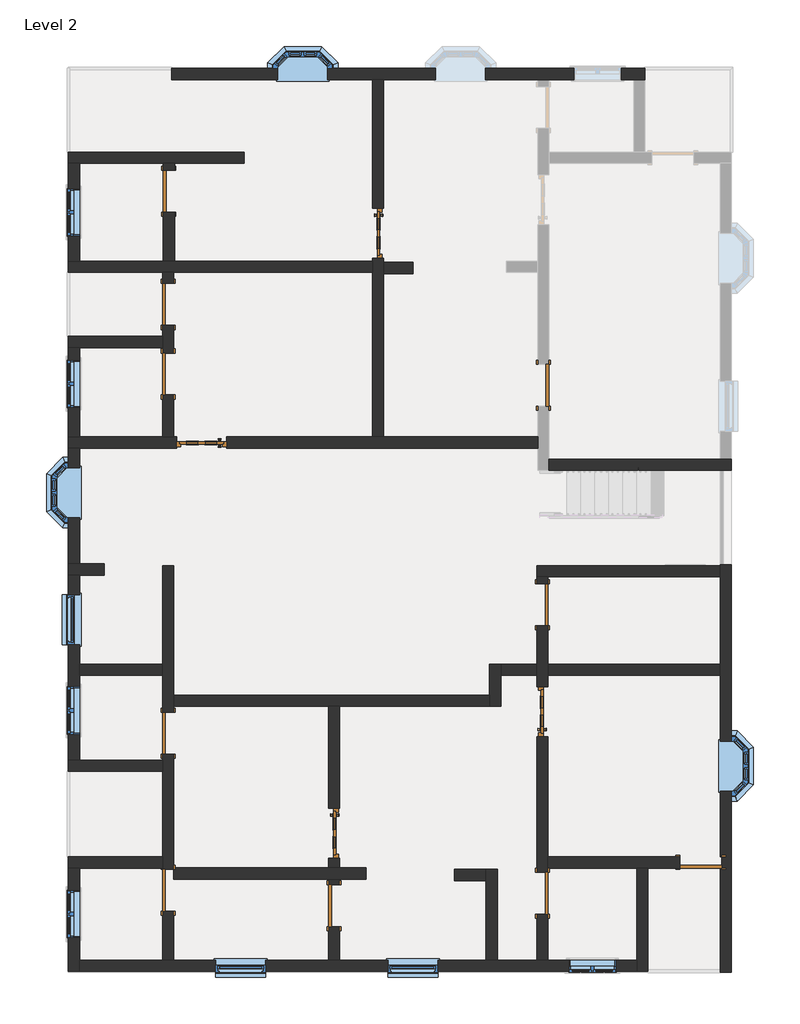
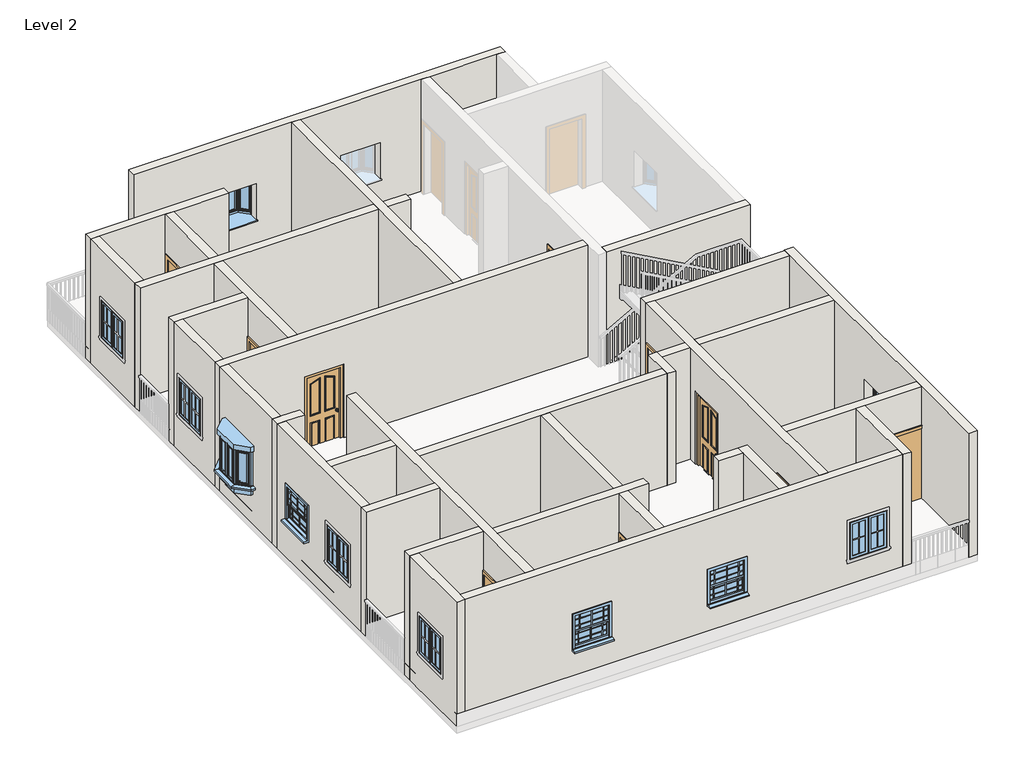
# One storey, part 1 of 4: 34 walls, 14 doors, 11 windows.
"""IFC4 building model written with IfcOpenShell, lengths in millimetres."""

from ifc_helpers import new_model, si_unit, frame, origin, place, context, project, spatial, polyline, outline, extrude, faceted_brep, transform, mapped, element, save
from components import doors_extsgl_12_910x2110mm_9a09825e, door_fadea3f2, door_53b1b562, window_910x910mm_67ef725a, window_c29befe5, windows_sash_w_bars_1_910x910mm_b688f793

model = new_model("IFC4")

# Units and contexts
model_context = context("Model", 3, world=origin())
ifc_project = project(units=[si_unit("LENGTHUNIT", "METRE", prefix="MILLI")], contexts=[model_context])

# Site, building, storey
site = spatial("IfcSite", under=ifc_project)
building = spatial("IfcBuilding", under=site)
storey = spatial("IfcBuildingStorey", under=building, Name="Level 2", Elevation=3048.0)

# Doors
placement = place(None, origin())
doors_extsgl_12_910x2110mm_shape = doors_extsgl_12_910x2110mm_9a09825e(model_context)
element("IfcDoor", 1, ObjectType="Doors_ExtSgl_12 : 910x2110mm", at=placement, inside=storey, context=model_context, shape_type="MappedRepresentation", body=[
    mapped(doors_extsgl_12_910x2110mm_shape, transform((-1409.2058717, 5320.2339901, 3048.0), x_axis=(0.0, -1.0, 0.0), y_axis=(1.0, 0.0, 0.0), z_axis=(0.0, 0.0, 1.0))),
])
element("IfcDoor", 2, ObjectType="Doors_ExtSgl_12 : 910x2110mm", at=placement, inside=storey, context=model_context, shape_type="MappedRepresentation", body=[
    mapped(doors_extsgl_12_910x2110mm_shape, transform((-4622.3058717, 1514.4547293, 3048.0), x_axis=(-1.0, 0.0, 0.0), y_axis=(0.0, -1.0, 0.0), z_axis=(0.0, 0.0, 1.0))),
])
element("IfcDoor", 3, ObjectType="Doors_ExtSgl_12 : 910x2110mm", at=placement, inside=storey, context=model_context, shape_type="MappedRepresentation", body=[
    mapped(doors_extsgl_12_910x2110mm_shape, transform((-2209.3058717, -5597.5452707, 3048.0), x_axis=(0.0, -1.0, 0.0), y_axis=(1.0, 0.0, 0.0), z_axis=(0.0, 0.0, 1.0))),
])
element("IfcDoor", 4, ObjectType="Doors_ExtSgl_12 : 910x2110mm", at=placement, inside=storey, context=model_context, shape_type="MappedRepresentation", body=[
    mapped(doors_extsgl_12_910x2110mm_shape, transform((1587.9941283, -3384.0437545, 3048.0), x_axis=(0.0, 1.0, 0.0), y_axis=(-1.0, 0.0, 0.0), z_axis=(0.0, 0.0, 1.0))),
])
door_shape = door_fadea3f2(model_context)
element("IfcDoor", 5, ObjectType="Single-Flush : 30\" x 80\"", at=placement, inside=storey, context=model_context, shape_type="MappedRepresentation", body=[
    mapped(door_shape, transform((-5219.2058717, 6086.4547293, 3048.0), x_axis=(0.0, 1.0, 0.0), y_axis=(-1.0, 0.0, 0.0), z_axis=(0.0, 0.0, 1.0))),
])
element("IfcDoor", 6, ObjectType="Single-Flush : 30\" x 80\"", at=placement, inside=storey, context=model_context, shape_type="MappedRepresentation", body=[
    mapped(door_shape, transform((-5231.9058717, -6637.2703483, 3048.0), x_axis=(0.0, 1.0, 0.0), y_axis=(-1.0, 0.0, 0.0), z_axis=(0.0, 0.0, 1.0))),
])
element("IfcDoor", 7, ObjectType="Single-Flush : 30\" x 80\"", at=placement, inside=storey, context=model_context, shape_type="MappedRepresentation", body=[
    mapped(door_shape, transform((-2209.3058717, -6918.3452707, 3048.0), x_axis=(0.0, 1.0, 0.0), y_axis=(-1.0, 0.0, 0.0), z_axis=(0.0, 0.0, 1.0))),
])
door_2_shape = door_53b1b562(model_context)
element("IfcDoor", 8, ObjectType="Single-Flush : 30\" x 80\"", at=placement, inside=storey, context=model_context, shape_type="MappedRepresentation", body=[
    mapped(door_2_shape, transform((-5231.9058717, 2759.0547293, 3048.0), x_axis=(0.0, -1.0, 0.0), y_axis=(1.0, 0.0, 0.0), z_axis=(0.0, 0.0, 1.0))),
])
element("IfcDoor", 9, ObjectType="Single-Flush : 30\" x 80\"", at=placement, inside=storey, context=model_context, shape_type="MappedRepresentation", body=[
    mapped(door_2_shape, transform((-5231.9058717, -3778.816952, 3048.0), x_axis=(0.0, -1.0, 0.0), y_axis=(1.0, 0.0, 0.0), z_axis=(0.0, 0.0, 1.0))),
])
element("IfcDoor", 10, ObjectType="Single-Flush : 30\" x 80\"", at=placement, inside=storey, context=model_context, shape_type="MappedRepresentation", body=[
    mapped(door_2_shape, transform((1587.9941283, -6689.7452707, 3048.0), x_axis=(0.0, 1.0, 0.0), y_axis=(-1.0, 0.0, 0.0), z_axis=(0.0, 0.0, 1.0))),
])
element("IfcDoor", 11, ObjectType="Single-Flush : 30\" x 80\"", at=placement, inside=storey, context=model_context, shape_type="MappedRepresentation", body=[
    mapped(door_2_shape, transform((4470.8941283, -6130.9452707, 3048.0), x_axis=(1.0, 0.0, 0.0), y_axis=(0.0, 1.0, 0.0), z_axis=(0.0, 0.0, 1.0))),
])
element("IfcDoor", 12, ObjectType="Single-Flush : 30\" x 80\"", at=placement, inside=storey, context=model_context, shape_type="MappedRepresentation", body=[
    mapped(door_2_shape, transform((1587.9941283, -1440.3867138, 3048.0), x_axis=(0.0, 1.0, 0.0), y_axis=(-1.0, 0.0, 0.0), z_axis=(0.0, 0.0, 1.0))),
])
element("IfcDoor", 13, ObjectType="Single-Flush : 30\" x 80\"", at=placement, inside=storey, context=model_context, shape_type="MappedRepresentation", body=[
    mapped(door_2_shape, transform((1600.6941283, 2555.8547293, 3048.0), x_axis=(0.0, 1.0, 0.0), y_axis=(-1.0, 0.0, 0.0), z_axis=(0.0, 0.0, 1.0))),
])
element("IfcDoor", 14, ObjectType="Single-Flush : 30\" x 80\"", at=placement, inside=storey, context=model_context, shape_type="MappedRepresentation", body=[
    mapped(door_2_shape, transform((-5231.9058717, 4026.9443597, 3048.0), x_axis=(0.0, -1.0, 0.0), y_axis=(1.0, 0.0, 0.0), z_axis=(0.0, 0.0, 1.0))),
])

# Walls
element("IfcWall", 15, ObjectType="Generic - 4.5\"", at=placement, inside=storey, context=model_context, shape_type="Brep", body=[
    faceted_brep([(-1510.8058717, 4865.2339901, 5158.0), (-1510.8058717, 4865.2339901, 3048.0), (-1510.8058717, 4812.2339901, 3048.0), (-1510.8058717, 4609.0339901, 3048.0), (-1510.8058717, 1616.0547293, 3048.0), (-1510.8058717, 1616.0547293, 6096.0), (-1510.8058717, 4609.0339901, 6096.0), (-1510.8058717, 4812.2339901, 6096.0), (-1510.8058717, 8118.4547293, 6096.0), (-1510.8058717, 8118.4547293, 3048.0), (-1510.8058717, 5775.2339901, 3048.0), (-1510.8058717, 5775.2339901, 5158.0), (-1307.6058717, 1616.0547293, 3048.0), (-1307.6058717, 4587.8547293, 3048.0), (-1307.6058717, 4791.0547293, 3048.0), (-1307.6058717, 4865.2339901, 3048.0), (-1307.6058717, 4865.2339901, 5158.0), (-1307.6058717, 5775.2339901, 5158.0), (-1307.6058717, 5775.2339901, 3048.0), (-1307.6058717, 8118.4547293, 3048.0), (-1307.6058717, 8118.4547293, 6096.0), (-1307.6058717, 4791.0547293, 6096.0), (-1307.6058717, 4587.8547293, 6096.0), (-1307.6058717, 1616.0547293, 6096.0)], [[[0, 1, 2, 3, 4, 5, 6, 7, 8, 9, 10, 11]], [[12, 13, 14, 15, 16, 17, 18, 19, 20, 21, 22, 23]], [[10, 9, 19, 18]], [[4, 3, 2, 1, 15, 14, 13, 12]], [[8, 7, 6, 5, 23, 22, 21, 20]], [[9, 8, 20, 19]], [[5, 4, 12, 23]], [[18, 17, 11, 10]], [[16, 15, 1, 0]], [[17, 16, 0, 11]]]),
])
element("IfcWall", 16, ObjectType="Generic - 4.5\"", at=placement, inside=storey, context=model_context, shape_type="Brep", body=[
    faceted_brep([(-7048.0058717, 4609.0339901, 3048.0), (-5333.5058717, 4609.0339901, 3048.0), (-5130.3058717, 4609.0339901, 3048.0), (-1510.8058717, 4609.0339901, 3048.0), (-1510.8058717, 4609.0339901, 6096.0), (-5130.3058717, 4609.0339901, 6096.0), (-5333.5058717, 4609.0339901, 6096.0), (-7048.0058717, 4609.0339901, 6096.0), (-7048.0058717, 4812.2339901, 3048.0), (-7048.0058717, 4812.2339901, 6096.0), (-6844.8058717, 4812.2339901, 6096.0), (-5320.8058717, 4812.2339901, 6096.0), (-5117.6058717, 4812.2339901, 6096.0), (-1510.8058717, 4812.2339901, 6096.0), (-1510.8058717, 4812.2339901, 3048.0), (-5117.6058717, 4812.2339901, 3048.0), (-5320.8058717, 4812.2339901, 3048.0), (-6844.8058717, 4812.2339901, 3048.0)], [[[0, 1, 2, 3, 4, 5, 6, 7]], [[8, 9, 10, 11, 12, 13, 14, 15, 16, 17]], [[3, 2, 1, 0, 8, 17, 16, 15, 14]], [[7, 6, 5, 4, 13, 12, 11, 10, 9]], [[4, 3, 14, 13]], [[0, 7, 9, 8]]]),
])
element("IfcWall", 17, ObjectType="Generic - 4.5\"", at=placement, inside=storey, context=model_context, shape_type="Brep", body=[
    faceted_brep([(-5333.5058717, 3645.9443597, 5080.0), (-5333.5058717, 3645.9443597, 3048.0), (-5333.5058717, 3444.8547293, 3048.0), (-5333.5058717, 3241.6547293, 3048.0), (-5333.5058717, 3140.0547293, 3048.0), (-5333.5058717, 3140.0547293, 5080.0), (-5333.5058717, 2378.0547293, 5080.0), (-5333.5058717, 2378.0547293, 3048.0), (-5333.5058717, 1616.0547293, 3048.0), (-5333.5058717, 1616.0547293, 6096.0), (-5333.5058717, 3241.6547293, 6096.0), (-5333.5058717, 3444.8547293, 6096.0), (-5333.5058717, 4609.0339901, 6096.0), (-5333.5058717, 4609.0339901, 3048.0), (-5333.5058717, 4407.9443597, 3048.0), (-5333.5058717, 4407.9443597, 5080.0), (-5130.3058717, 3140.0547293, 3048.0), (-5130.3058717, 3645.9443597, 3048.0), (-5130.3058717, 3645.9443597, 5080.0), (-5130.3058717, 4407.9443597, 5080.0), (-5130.3058717, 4407.9443597, 3048.0), (-5130.3058717, 4609.0339901, 3048.0), (-5130.3058717, 4609.0339901, 6096.0), (-5130.3058717, 1616.0547293, 6096.0), (-5130.3058717, 1616.0547293, 3048.0), (-5130.3058717, 2378.0547293, 3048.0), (-5130.3058717, 2378.0547293, 5080.0), (-5130.3058717, 3140.0547293, 5080.0)], [[[0, 1, 2, 3, 4, 5, 6, 7, 8, 9, 10, 11, 12, 13, 14, 15]], [[16, 17, 18, 19, 20, 21, 22, 23, 24, 25, 26, 27]], [[8, 7, 25, 24]], [[14, 13, 21, 20]], [[4, 3, 2, 1, 17, 16]], [[12, 11, 10, 9, 23, 22]], [[13, 12, 22, 21]], [[9, 8, 24, 23]], [[26, 25, 7, 6]], [[27, 26, 6, 5]], [[16, 27, 5, 4]], [[18, 17, 1, 0]], [[19, 18, 0, 15]], [[20, 19, 15, 14]]]),
])
element("IfcWall", 18, ObjectType="Generic - 4.5\"", at=placement, inside=storey, context=model_context, shape_type="Brep", body=[
    faceted_brep([(-5130.3058717, -6256.2703483, 5080.0), (-5130.3058717, -6256.2703483, 3048.0), (-5130.3058717, -6230.8703483, 3048.0), (-5130.3058717, -4159.816952, 3048.0), (-5130.3058717, -4159.816952, 5080.0), (-5130.3058717, -3397.816952, 5080.0), (-5130.3058717, -3397.816952, 3048.0), (-5130.3058717, -3286.1452707, 3048.0), (-5130.3058717, -3082.9452707, 3048.0), (-5130.3058717, -733.4452707, 3048.0), (-5130.3058717, -733.4452707, 6096.0), (-5130.3058717, -3082.9452707, 6096.0), (-5130.3058717, -3286.1452707, 6096.0), (-5130.3058717, -6230.8703483, 6096.0), (-5130.3058717, -6434.0703483, 6096.0), (-5130.3058717, -7908.9452707, 6096.0), (-5130.3058717, -7908.9452707, 3048.0), (-5130.3058717, -7018.2703483, 3048.0), (-5130.3058717, -7018.2703483, 5080.0), (-5333.5058717, -4159.816952, 3048.0), (-5333.5058717, -4271.4886333, 3048.0), (-5333.5058717, -4474.6886333, 3048.0), (-5333.5058717, -6029.3452707, 3048.0), (-5333.5058717, -6232.5452707, 3048.0), (-5333.5058717, -6256.2703483, 3048.0), (-5333.5058717, -6256.2703483, 5080.0), (-5333.5058717, -7018.2703483, 5080.0), (-5333.5058717, -7018.2703483, 3048.0), (-5333.5058717, -7908.9452707, 3048.0), (-5333.5058717, -7908.9452707, 6096.0), (-5333.5058717, -6232.5452707, 6096.0), (-5333.5058717, -6029.3452707, 6096.0), (-5333.5058717, -4474.6886333, 6096.0), (-5333.5058717, -4271.4886333, 6096.0), (-5333.5058717, -2727.3452707, 6096.0), (-5333.5058717, -2524.1452707, 6096.0), (-5333.5058717, -733.4452707, 6096.0), (-5333.5058717, -733.4452707, 3048.0), (-5333.5058717, -2524.1452707, 3048.0), (-5333.5058717, -2727.3452707, 3048.0), (-5333.5058717, -3397.816952, 3048.0), (-5333.5058717, -3397.816952, 5080.0), (-5333.5058717, -4159.816952, 5080.0)], [[[0, 1, 2, 3, 4, 5, 6, 7, 8, 9, 10, 11, 12, 13, 14, 15, 16, 17, 18]], [[19, 20, 21, 22, 23, 24, 25, 26, 27, 28, 29, 30, 31, 32, 33, 34, 35, 36, 37, 38, 39, 40, 41, 42]], [[40, 39, 38, 37, 9, 8, 7, 6]], [[17, 16, 28, 27]], [[3, 2, 1, 24, 23, 22, 21, 20, 19]], [[10, 9, 37, 36]], [[15, 14, 13, 12, 11, 10, 36, 35, 34, 33, 32, 31, 30, 29]], [[4, 3, 19, 42]], [[5, 4, 42, 41]], [[6, 5, 41, 40]], [[25, 24, 1, 0]], [[26, 25, 0, 18]], [[27, 26, 18, 17]], [[16, 15, 29, 28]]]),
])
element("IfcWall", 19, ObjectType="Generic - 4.5\"", at=placement, inside=storey, context=model_context, shape_type="Brep", body=[
    faceted_brep([(-7048.0058717, -898.5452707, 3048.0), (-6844.8058717, -898.5452707, 3048.0), (-6400.7404065, -898.5452707, 3048.0), (-6400.7404065, -898.5452707, 6096.0), (-6844.8058717, -898.5452707, 6096.0), (-7048.0058717, -898.5452707, 6096.0), (-7048.0058717, -695.3452707, 3048.0), (-7048.0058717, -695.3452707, 6096.0), (-6844.8058717, -695.3452707, 6096.0), (-6400.7404065, -695.3452707, 6096.0), (-6400.7404065, -695.3452707, 3048.0), (-6844.8058717, -695.3452707, 3048.0)], [[[0, 1, 2, 3, 4, 5]], [[6, 7, 8, 9, 10, 11]], [[2, 1, 0, 6, 11, 10]], [[3, 2, 10, 9]], [[5, 4, 3, 9, 8, 7]], [[0, 5, 7, 6]]]),
])
element("IfcWall", 20, ObjectType="Generic - 4.5\"", at=placement, inside=storey, context=model_context, shape_type="Brep", body=[
    faceted_brep([(-7048.0058717, 6594.4547293, 3048.0), (-6844.8058717, 6594.4547293, 3048.0), (-5320.8058717, 6594.4547293, 3048.0), (-5117.6058717, 6594.4547293, 3048.0), (-3847.6058717, 6594.4547293, 3048.0), (-3847.6058717, 6594.4547293, 6096.0), (-5117.6058717, 6594.4547293, 6096.0), (-5320.8058717, 6594.4547293, 6096.0), (-6844.8058717, 6594.4547293, 6096.0), (-7048.0058717, 6594.4547293, 6096.0), (-7048.0058717, 6797.6547293, 3048.0), (-7048.0058717, 6797.6547293, 6096.0), (-3847.6058717, 6797.6547293, 6096.0), (-3847.6058717, 6797.6547293, 3048.0)], [[[0, 1, 2, 3, 4, 5, 6, 7, 8, 9]], [[10, 11, 12, 13]], [[4, 3, 2, 1, 0, 10, 13]], [[5, 4, 13, 12]], [[9, 8, 7, 6, 5, 12, 11]], [[0, 9, 11, 10]]]),
])
element("IfcWall", 21, ObjectType="Generic - 4.5\"", at=placement, inside=storey, context=model_context, shape_type="Brep", body=[
    faceted_brep([(-7048.0058717, 3241.6547293, 3048.0), (-6844.8058717, 3241.6547293, 3048.0), (-5333.5058717, 3241.6547293, 3048.0), (-5333.5058717, 3241.6547293, 6096.0), (-6844.8058717, 3241.6547293, 6096.0), (-7048.0058717, 3241.6547293, 6096.0), (-7048.0058717, 3444.8547293, 3048.0), (-7048.0058717, 3444.8547293, 6096.0), (-5333.5058717, 3444.8547293, 6096.0), (-5333.5058717, 3444.8547293, 3048.0)], [[[0, 1, 2, 3, 4, 5]], [[6, 7, 8, 9]], [[2, 1, 0, 6, 9]], [[5, 4, 3, 8, 7]], [[3, 2, 9, 8]], [[0, 5, 7, 6]]]),
])
element("IfcWall", 22, ObjectType="Generic - 4.5\"", at=placement, inside=storey, context=model_context, shape_type="Brep", body=[
    faceted_brep([(-7048.0058717, 1412.8547293, 3048.0), (-6844.8058717, 1412.8547293, 3048.0), (-5077.3058717, 1412.8547293, 3048.0), (-5077.3058717, 1412.8547293, 5158.0), (-4167.3058717, 1412.8547293, 5158.0), (-4167.3058717, 1412.8547293, 3048.0), (1499.0941283, 1412.8547293, 3048.0), (1499.0941283, 1412.8547293, 6096.0), (-6844.8058717, 1412.8547293, 6096.0), (-7048.0058717, 1412.8547293, 6096.0), (-5077.3058717, 1616.0547293, 5158.0), (-5077.3058717, 1616.0547293, 3048.0), (-5130.3058717, 1616.0547293, 3048.0), (-5333.5058717, 1616.0547293, 3048.0), (-6844.8058717, 1616.0547293, 3048.0), (-7048.0058717, 1616.0547293, 3048.0), (-7048.0058717, 1616.0547293, 6096.0), (-6844.8058717, 1616.0547293, 6096.0), (-5333.5058717, 1616.0547293, 6096.0), (-5130.3058717, 1616.0547293, 6096.0), (-1510.8058717, 1616.0547293, 6096.0), (-1307.6058717, 1616.0547293, 6096.0), (1499.0941283, 1616.0547293, 6096.0), (1499.0941283, 1616.0547293, 3048.0), (-1307.6058717, 1616.0547293, 3048.0), (-1510.8058717, 1616.0547293, 3048.0), (-4167.3058717, 1616.0547293, 3048.0), (-4167.3058717, 1616.0547293, 5158.0)], [[[0, 1, 2, 3, 4, 5, 6, 7, 8, 9]], [[10, 11, 12, 13, 14, 15, 16, 17, 18, 19, 20, 21, 22, 23, 24, 25, 26, 27]], [[26, 25, 24, 23, 6, 5]], [[15, 14, 13, 12, 11, 2, 1, 0]], [[9, 8, 7, 22, 21, 20, 19, 18, 17, 16]], [[7, 6, 23, 22]], [[5, 4, 27, 26]], [[3, 2, 11, 10]], [[4, 3, 10, 27]], [[0, 9, 16, 15]]]),
])
element("IfcWall", 23, ObjectType="Generic - 4.5\"", at=placement, inside=storey, context=model_context, shape_type="Brep", body=[
    faceted_brep([(1702.2941283, 1006.4547293, 3048.0), (5029.6941283, 1006.4547293, 3048.0), (5029.6941283, 1006.4547293, 6096.0), (1702.2941283, 1006.4547293, 6096.0), (1702.2941283, 1209.6547293, 3048.0), (1702.2941283, 1209.6547293, 6096.0), (4826.4941283, 1209.6547293, 6096.0), (5029.6941283, 1209.6547293, 6096.0), (5029.6941283, 1209.6547293, 3048.0), (4826.4941283, 1209.6547293, 3048.0)], [[[0, 1, 2, 3]], [[4, 5, 6, 7, 8, 9]], [[1, 0, 4, 9, 8]], [[3, 2, 7, 6, 5]], [[0, 3, 5, 4]], [[2, 1, 8, 7]]]),
])
element("IfcWall", 24, ObjectType="Generic - 4.5\"", at=placement, inside=storey, context=model_context, shape_type="Brep", body=[
    faceted_brep([(1486.3941283, -932.3867138, 3048.0), (1689.5941283, -932.3867138, 3048.0), (4826.4941283, -932.3867138, 3048.0), (4826.4941283, -932.3867138, 6096.0), (1689.5941283, -932.3867138, 6096.0), (1486.3941283, -932.3867138, 6096.0), (1486.3941283, -729.1867138, 3048.0), (1486.3941283, -729.1867138, 6096.0), (4826.4941283, -729.1867138, 6096.0), (4826.4941283, -729.1867138, 3048.0)], [[[0, 1, 2, 3, 4, 5]], [[6, 7, 8, 9]], [[2, 1, 0, 6, 9]], [[5, 4, 3, 8, 7]], [[3, 2, 9, 8]], [[0, 5, 7, 6]]]),
])
element("IfcWall", 25, ObjectType="Generic - 4.5\"", at=placement, inside=storey, context=model_context, shape_type="Brep", body=[
    faceted_brep([(1486.3941283, -932.3867138, 3048.0), (1486.3941283, -1059.3867138, 3048.0), (1486.3941283, -1059.3867138, 5080.0), (1486.3941283, -1821.3867138, 5080.0), (1486.3941283, -1821.3867138, 3048.0), (1486.3941283, -2520.4437545, 3048.0), (1486.3941283, -2723.6437545, 3048.0), (1486.3941283, -2929.0437545, 3048.0), (1486.3941283, -2929.0437545, 5158.0), (1486.3941283, -3839.0437545, 5158.0), (1486.3941283, -3839.0437545, 3048.0), (1486.3941283, -6308.7452707, 3048.0), (1486.3941283, -6308.7452707, 5080.0), (1486.3941283, -7070.7452707, 5080.0), (1486.3941283, -7070.7452707, 3048.0), (1486.3941283, -7908.9452707, 3048.0), (1486.3941283, -7908.9452707, 6096.0), (1486.3941283, -2723.6437545, 6096.0), (1486.3941283, -2520.4437545, 6096.0), (1486.3941283, -932.3867138, 6096.0), (1689.5941283, -1059.3867138, 5080.0), (1689.5941283, -1059.3867138, 3048.0), (1689.5941283, -932.3867138, 3048.0), (1689.5941283, -932.3867138, 6096.0), (1689.5941283, -2520.4437545, 6096.0), (1689.5941283, -2723.6437545, 6096.0), (1689.5941283, -6029.3452707, 6096.0), (1689.5941283, -6232.5452707, 6096.0), (1689.5941283, -7908.9452707, 6096.0), (1689.5941283, -7908.9452707, 3048.0), (1689.5941283, -7070.7452707, 3048.0), (1689.5941283, -7070.7452707, 5080.0), (1689.5941283, -6308.7452707, 5080.0), (1689.5941283, -6308.7452707, 3048.0), (1689.5941283, -6232.5452707, 3048.0), (1689.5941283, -6029.3452707, 3048.0), (1689.5941283, -3839.0437545, 3048.0), (1689.5941283, -3839.0437545, 5158.0), (1689.5941283, -2929.0437545, 5158.0), (1689.5941283, -2929.0437545, 3048.0), (1689.5941283, -2723.6437545, 3048.0), (1689.5941283, -2520.4437545, 3048.0), (1689.5941283, -1821.3867138, 3048.0), (1689.5941283, -1821.3867138, 5080.0)], [[[0, 1, 2, 3, 4, 5, 6, 7, 8, 9, 10, 11, 12, 13, 14, 15, 16, 17, 18, 19]], [[20, 21, 22, 23, 24, 25, 26, 27, 28, 29, 30, 31, 32, 33, 34, 35, 36, 37, 38, 39, 40, 41, 42, 43]], [[30, 29, 15, 14]], [[36, 35, 34, 33, 11, 10]], [[22, 21, 1, 0]], [[42, 41, 40, 39, 7, 6, 5, 4]], [[19, 18, 17, 16, 28, 27, 26, 25, 24, 23]], [[0, 19, 23, 22]], [[10, 9, 37, 36]], [[8, 7, 39, 38]], [[9, 8, 38, 37]], [[12, 11, 33, 32]], [[13, 12, 32, 31]], [[14, 13, 31, 30]], [[2, 1, 21, 20]], [[3, 2, 20, 43]], [[4, 3, 43, 42]], [[16, 15, 29, 28]]]),
])
element("IfcWall", 26, ObjectType="Generic - 4.5\"", at=placement, inside=storey, context=model_context, shape_type="SweptSolid", body=[
    extrude(outline(polyline([(4826.4941283, -2723.6437545), (1689.5941283, -2723.6437545), (1689.5941283, -2520.4437545), (4826.4941283, -2520.4437545), (4826.4941283, -2723.6437545)])), frame((0.0, 0.0, 3048.0), z_axis=(0.0, 0.0, 1.0), x_axis=(1.0, 0.0, 0.0)), (0.0, 0.0, 1.0), 3048.0),
])
element("IfcWall", 27, ObjectType="Generic - 4.5\"", at=placement, inside=storey, context=model_context, shape_type="Brep", body=[
    faceted_brep([(4826.4941283, -6232.5452707, 6096.0), (3505.6941283, -6232.5452707, 6096.0), (3302.4941283, -6232.5452707, 6096.0), (1689.5941283, -6232.5452707, 6096.0), (1689.5941283, -6232.5452707, 3048.0), (3302.4941283, -6232.5452707, 3048.0), (3505.6941283, -6232.5452707, 3048.0), (4089.8941283, -6232.5452707, 3048.0), (4089.8941283, -6232.5452707, 5080.0), (4826.4941283, -6232.5452707, 5080.0), (1689.5941283, -6029.3452707, 6096.0), (4826.4941283, -6029.3452707, 6096.0), (4826.4941283, -6029.3452707, 5080.0), (4089.8941283, -6029.3452707, 5080.0), (4089.8941283, -6029.3452707, 3048.0), (1689.5941283, -6029.3452707, 3048.0)], [[[0, 1, 2, 3, 4, 5, 6, 7, 8, 9]], [[10, 11, 12, 13, 14, 15]], [[4, 15, 14, 7, 6, 5]], [[3, 2, 1, 0, 11, 10]], [[11, 0, 9, 12]], [[4, 3, 10, 15]], [[8, 13, 12, 9]], [[13, 8, 7, 14]]]),
])
element("IfcWall", 28, ObjectType="Generic - 4.5\"", at=placement, inside=storey, context=model_context, shape_type="Brep", body=[
    faceted_brep([(3302.4941283, -6232.5452707, 3048.0), (3302.4941283, -7908.9452707, 3048.0), (3302.4941283, -8112.1452707, 3048.0), (3302.4941283, -8112.1452707, 6096.0), (3302.4941283, -7908.9452707, 6096.0), (3302.4941283, -6232.5452707, 6096.0), (3505.6941283, -6232.5452707, 3048.0), (3505.6941283, -6232.5452707, 6096.0), (3505.6941283, -8112.1452707, 6096.0), (3505.6941283, -8112.1452707, 3048.0)], [[[0, 1, 2, 3, 4, 5]], [[6, 7, 8, 9]], [[2, 1, 0, 6, 9]], [[5, 4, 3, 8, 7]], [[0, 5, 7, 6]], [[3, 2, 9, 8]]]),
])
element("IfcWall", 29, ObjectType="Generic - 4.5\"", at=placement, inside=storey, context=model_context, shape_type="SweptSolid", body=[
    extrude(outline(polyline([(-5333.5058717, -2727.3452707), (-6844.8058717, -2727.3452707), (-6844.8058717, -2524.1452707), (-5333.5058717, -2524.1452707), (-5333.5058717, -2727.3452707)])), frame((0.0, 0.0, 3048.0), z_axis=(0.0, 0.0, 1.0), x_axis=(1.0, 0.0, 0.0)), (0.0, 0.0, 1.0), 3048.0),
])
element("IfcWall", 30, ObjectType="Generic - 4.5\"", at=placement, inside=storey, context=model_context, shape_type="Brep", body=[
    faceted_brep([(-7048.0058717, -4474.6886333, 3048.0), (-5333.5058717, -4474.6886333, 3048.0), (-5333.5058717, -4474.6886333, 6096.0), (-7048.0058717, -4474.6886333, 6096.0), (-7048.0058717, -4271.4886333, 3048.0), (-7048.0058717, -4271.4886333, 6096.0), (-6844.8058717, -4271.4886333, 6096.0), (-5333.5058717, -4271.4886333, 6096.0), (-5333.5058717, -4271.4886333, 3048.0), (-6844.8058717, -4271.4886333, 3048.0)], [[[0, 1, 2, 3]], [[4, 5, 6, 7, 8, 9]], [[1, 0, 4, 9, 8]], [[3, 2, 7, 6, 5]], [[2, 1, 8, 7]], [[0, 3, 5, 4]]]),
])
element("IfcWall", 31, ObjectType="Generic - 4.5\"", at=placement, inside=storey, context=model_context, shape_type="Brep", body=[
    faceted_brep([(-7048.0058717, -6232.5452707, 3048.0), (-6844.8058717, -6232.5452707, 3048.0), (-5333.5058717, -6232.5452707, 3048.0), (-5333.5058717, -6232.5452707, 6096.0), (-6844.8058717, -6232.5452707, 6096.0), (-7048.0058717, -6232.5452707, 6096.0), (-7048.0058717, -6029.3452707, 3048.0), (-7048.0058717, -6029.3452707, 6096.0), (-5333.5058717, -6029.3452707, 6096.0), (-5333.5058717, -6029.3452707, 3048.0)], [[[0, 1, 2, 3, 4, 5]], [[6, 7, 8, 9]], [[2, 1, 0, 6, 9]], [[5, 4, 3, 8, 7]], [[3, 2, 9, 8]], [[0, 5, 7, 6]]]),
])
element("IfcWall", 32, ObjectType="Generic - 4.5\"", at=placement, inside=storey, context=model_context, shape_type="Brep", body=[
    faceted_brep([(-5130.3058717, -6434.0703483, 3048.0), (-2310.9058717, -6434.0703483, 3048.0), (-2107.7058717, -6434.0703483, 3048.0), (-1625.1058717, -6434.0703483, 3048.0), (-1625.1058717, -6434.0703483, 6096.0), (-2107.7058717, -6434.0703483, 6096.0), (-2310.9058717, -6434.0703483, 6096.0), (-5130.3058717, -6434.0703483, 6096.0), (-5130.3058717, -6230.8703483, 3048.0), (-5130.3058717, -6230.8703483, 6096.0), (-2310.9058717, -6230.8703483, 6096.0), (-2107.7058717, -6230.8703483, 6096.0), (-1625.1058717, -6230.8703483, 6096.0), (-1625.1058717, -6230.8703483, 3048.0), (-2107.7058717, -6230.8703483, 3048.0), (-2310.9058717, -6230.8703483, 3048.0), (-5130.3058717, -6256.2703483, 3048.0)], [[[0, 1, 2, 3, 4, 5, 6, 7]], [[8, 9, 10, 11, 12, 13, 14, 15]], [[3, 2, 1, 0, 16, 8, 15, 14, 13]], [[4, 3, 13, 12]], [[7, 6, 5, 4, 12, 11, 10, 9]], [[0, 7, 9, 8, 16]]]),
])
element("IfcWall", 33, ObjectType="Generic - 4.5\"", at=placement, inside=storey, context=model_context, shape_type="Brep", body=[
    faceted_brep([(762.4941283, -7908.9452707, 3048.0), (762.4941283, -6257.9452707, 3048.0), (762.4941283, -6257.9452707, 6096.0), (762.4941283, -7908.9452707, 6096.0), (559.2941283, -7908.9452707, 3048.0), (559.2941283, -7908.9452707, 6096.0), (559.2941283, -6461.1452707, 6096.0), (559.2941283, -6257.9452707, 6096.0), (559.2941283, -6257.9452707, 3048.0), (559.2941283, -6461.1452707, 3048.0)], [[[0, 1, 2, 3]], [[4, 5, 6, 7, 8, 9]], [[1, 0, 4, 9, 8]], [[3, 2, 7, 6, 5]], [[2, 1, 8, 7]], [[0, 3, 5, 4]]]),
])
element("IfcWall", 34, ObjectType="Generic - 4.5\"", at=placement, inside=storey, context=model_context, shape_type="SweptSolid", body=[
    extrude(outline(polyline([(-12.2058717, -6257.9452707), (559.2941283, -6257.9452707), (559.2941283, -6461.1452707), (-12.2058717, -6461.1452707), (-12.2058717, -6257.9452707)])), frame((0.0, 0.0, 3048.0), z_axis=(0.0, 0.0, 1.0), x_axis=(1.0, 0.0, 0.0)), (0.0, 0.0, 1.0), 3048.0),
])
element("IfcWall", 35, ObjectType="Generic - 4.5\"", at=placement, inside=storey, context=model_context, shape_type="SweptSolid", body=[
    extrude(outline(polyline([(-3286.1452707, 6096.0), (-3286.1452707, 3048.0), (-5142.5452707, 3048.0), (-5142.5452707, 5158.0), (-6052.5452707, 5158.0), (-6052.5452707, 3048.0), (-6230.8703483, 3048.0), (-6230.8703483, 6096.0), (-3286.1452707, 6096.0)])), frame((-2310.9058717, 0.0, 0.0), z_axis=(1.0, 0.0, 0.0), x_axis=(0.0, 1.0, 0.0)), (0.0, 0.0, 1.0), 203.2),
    extrude(outline(polyline([(-6537.3452707, 3048.0), (-6537.3452707, 5080.0), (-7299.3452707, 5080.0), (-7299.3452707, 3048.0), (-7908.9452707, 3048.0), (-7908.9452707, 6096.0), (-6434.0703483, 6096.0), (-6434.0703483, 3048.0), (-6537.3452707, 3048.0)])), frame((-2310.9058717, 0.0, 0.0), z_axis=(1.0, 0.0, 0.0), x_axis=(0.0, 1.0, 0.0)), (0.0, 0.0, 1.0), 203.2),
])
element("IfcWall", 36, ObjectType="Generic - 4.5\"", at=placement, inside=storey, context=model_context, shape_type="Brep", body=[
    faceted_brep([(-5130.3058717, -3286.1452707, 3048.0), (-2310.9058717, -3286.1452707, 3048.0), (-2107.7058717, -3286.1452707, 3048.0), (622.0199378, -3286.1452707, 3048.0), (622.0199378, -3286.1452707, 6096.0), (-2107.7058717, -3286.1452707, 6096.0), (-2310.9058717, -3286.1452707, 6096.0), (-5130.3058717, -3286.1452707, 6096.0), (-5130.3058717, -3082.9452707, 3048.0), (-5130.3058717, -3082.9452707, 6096.0), (622.0199378, -3082.9452707, 6096.0), (622.0199378, -3082.9452707, 3048.0)], [[[0, 1, 2, 3, 4, 5, 6, 7]], [[8, 9, 10, 11]], [[3, 2, 1, 0, 8, 11]], [[7, 6, 5, 4, 10, 9]], [[0, 7, 9, 8]], [[4, 3, 11, 10]]]),
])
element("IfcWall", 37, ObjectType="Generic - 4.5\"", at=placement, inside=storey, context=model_context, shape_type="Brep", body=[
    faceted_brep([(825.2199378, -3286.1452707, 3048.0), (825.2199378, -2723.6437545, 3048.0), (825.2199378, -2520.4437545, 3048.0), (825.2199378, -2520.4437545, 6096.0), (825.2199378, -2723.6437545, 6096.0), (825.2199378, -3286.1452707, 6096.0), (622.0199378, -3286.1452707, 3048.0), (622.0199378, -3286.1452707, 6096.0), (622.0199378, -3082.9452707, 6096.0), (622.0199378, -2520.4437545, 6096.0), (622.0199378, -2520.4437545, 3048.0), (622.0199378, -3082.9452707, 3048.0)], [[[0, 1, 2, 3, 4, 5]], [[6, 7, 8, 9, 10, 11]], [[2, 1, 0, 6, 11, 10]], [[5, 4, 3, 9, 8, 7]], [[0, 5, 7, 6]], [[3, 2, 10, 9]]]),
])
element("IfcWall", 38, ObjectType="Generic - 4.5\"", at=placement, inside=storey, context=model_context, shape_type="SweptSolid", body=[
    extrude(outline(polyline([(1486.3941283, -2723.6437545), (825.2199378, -2723.6437545), (825.2199378, -2520.4437545), (1486.3941283, -2520.4437545), (1486.3941283, -2723.6437545)])), frame((0.0, 0.0, 3048.0), z_axis=(0.0, 0.0, 1.0), x_axis=(1.0, 0.0, 0.0)), (0.0, 0.0, 1.0), 3048.0),
])
element("IfcWall", 39, ObjectType="Generic - 4.5\"", at=placement, inside=storey, context=model_context, shape_type="SweptSolid", body=[
    extrude(outline(polyline([(-774.2058717, 4587.8547293), (-1307.6058717, 4587.8547293), (-1307.6058717, 4791.0547293), (-774.2058717, 4791.0547293), (-774.2058717, 4587.8547293)])), frame((0.0, 0.0, 3048.0), z_axis=(0.0, 0.0, 1.0), x_axis=(1.0, 0.0, 0.0)), (0.0, 0.0, 1.0), 3048.0),
])
element("IfcWall", 40, ObjectType="Generic - 4.5\"", at=placement, inside=storey, context=model_context, shape_type="SweptSolid", body=[
    extrude(outline(polyline([(6594.4547293, 3048.0), (6467.4547293, 3048.0), (6467.4547293, 5080.0), (5705.4547293, 5080.0), (5705.4547293, 3048.0), (4812.2339901, 3048.0), (4812.2339901, 6096.0), (6594.4547293, 6096.0), (6594.4547293, 3048.0)])), frame((-5320.8058717, 0.0, 0.0), z_axis=(1.0, 0.0, 0.0), x_axis=(0.0, 1.0, 0.0)), (0.0, 0.0, 1.0), 203.2),
])
element("IfcWall", 41, ObjectType="Generic - 9\"", at=placement, inside=storey, context=model_context, shape_type="Brep", body=[
    faceted_brep([(-5168.4058717, 8118.4547293, 3048.0), (-1510.8058717, 8118.4547293, 3048.0), (-1307.6058717, 8118.4547293, 3048.0), (1499.0941283, 8118.4547293, 3048.0), (1702.2941283, 8118.4547293, 3048.0), (3251.6941283, 8118.4547293, 3048.0), (3454.8941283, 8118.4547293, 3048.0), (3454.8941283, 8118.4547293, 6096.0), (3251.6941283, 8118.4547293, 6096.0), (1702.2941283, 8118.4547293, 6096.0), (1499.0941283, 8118.4547293, 6096.0), (-1307.6058717, 8118.4547293, 6096.0), (-1510.8058717, 8118.4547293, 6096.0), (-5168.4058717, 8118.4547293, 6096.0), (-359.2558717, 8118.4547293, 4872.4), (550.7441283, 8118.4547293, 4872.4), (550.7441283, 8118.4547293, 3962.4), (-359.2558717, 8118.4547293, 3962.4), (-3235.8058717, 8118.4547293, 4872.4), (-2325.8058717, 8118.4547293, 4872.4), (-2325.8058717, 8118.4547293, 3962.4), (-3235.8058717, 8118.4547293, 3962.4), (3023.0941283, 8118.4547293, 4876.8), (3023.0941283, 8118.4547293, 3962.4), (2159.4941283, 8118.4547293, 3962.4), (2159.4941283, 8118.4547293, 4876.8), (-5168.4058717, 8321.6547293, 3048.0), (-5168.4058717, 8321.6547293, 6096.0), (3454.8941283, 8321.6547293, 6096.0), (3454.8941283, 8321.6547293, 3048.0), (-359.2558717, 8321.6547293, 4872.4), (-359.2558717, 8321.6547293, 3962.4), (550.7441283, 8321.6547293, 3962.4), (550.7441283, 8321.6547293, 4872.4), (-3235.8058717, 8321.6547293, 4872.4), (-3235.8058717, 8321.6547293, 3962.4), (-2325.8058717, 8321.6547293, 3962.4), (-2325.8058717, 8321.6547293, 4872.4), (3023.0941283, 8321.6547293, 4876.8), (2159.4941283, 8321.6547293, 4876.8), (2159.4941283, 8321.6547293, 3962.4), (3023.0941283, 8321.6547293, 3962.4)], [[[0, 1, 2, 3, 4, 5, 6, 7, 8, 9, 10, 11, 12, 13], [14, 15, 16, 17], [18, 19, 20, 21], [22, 23, 24, 25]], [[26, 27, 28, 29], [30, 31, 32, 33], [34, 35, 36, 37], [38, 39, 40, 41]], [[6, 5, 4, 3, 2, 1, 0, 26, 29]], [[13, 12, 11, 10, 9, 8, 7, 28, 27]], [[0, 13, 27, 26]], [[31, 30, 14, 17]], [[32, 31, 17, 16]], [[33, 32, 16, 15]], [[30, 33, 15, 14]], [[35, 34, 18, 21]], [[36, 35, 21, 20]], [[37, 36, 20, 19]], [[34, 37, 19, 18]], [[23, 22, 38, 41]], [[24, 23, 41, 40]], [[25, 24, 40, 39]], [[22, 25, 39, 38]], [[7, 6, 29, 28]]]),
])
element("IfcWall", 42, ObjectType="Generic - 9\"", at=placement, inside=storey, context=model_context, shape_type="Brep", body=[
    faceted_brep([(4826.4941283, -8124.8452707, 3048.0), (4826.4941283, -8124.8452707, 6096.0), (4826.4941283, -6232.5452707, 6096.0), (4826.4941283, -6029.3452707, 6096.0), (4826.4941283, -2723.6437545, 6096.0), (4826.4941283, -2520.4437545, 6096.0), (4826.4941283, -932.3867138, 6096.0), (4826.4941283, -729.1867138, 6096.0), (4826.4941283, -714.2964201, 6096.0), (4826.4941283, -714.2964201, 3048.0), (4826.4941283, -729.1867138, 3048.0), (4826.4941283, -932.3867138, 3048.0), (4826.4941283, -2520.4437545, 3048.0), (4826.4941283, -2723.6437545, 3048.0), (4826.4941283, -6029.3452707, 3048.0), (4826.4941283, -6029.3452707, 5080.0), (4826.4941283, -6232.5452707, 5080.0), (4826.4941283, -6232.5452707, 3048.0), (4826.4941283, -3921.4945126, 4872.4), (4826.4941283, -4831.4945126, 4872.4), (4826.4941283, -4831.4945126, 3962.4), (4826.4941283, -3921.4945126, 3962.4), (5029.6941283, -8124.8452707, 3048.0), (5029.6941283, -714.2964201, 3048.0), (5029.6941283, -714.2964201, 6096.0), (5029.6941283, -8124.8452707, 6096.0), (5029.6941283, -3921.4945126, 4872.4), (5029.6941283, -3921.4945126, 3962.4), (5029.6941283, -4831.4945126, 3962.4), (5029.6941283, -4831.4945126, 4872.4), (4851.8941283, -6232.5452707, 3048.0), (4851.8941283, -6029.3452707, 3048.0), (4851.8941283, -6232.5452707, 5080.0), (4851.8941283, -6029.3452707, 5080.0)], [[[0, 1, 2, 3, 4, 5, 6, 7, 8, 9, 10, 11, 12, 13, 14, 15, 16, 17], [18, 19, 20, 21]], [[22, 23, 24, 25], [26, 27, 28, 29]], [[23, 22, 0, 17, 30, 31, 14, 13, 12, 11, 10, 9]], [[1, 0, 22, 25]], [[8, 7, 6, 5, 4, 3, 2, 1, 25, 24]], [[9, 8, 24, 23]], [[32, 30, 17, 16]], [[31, 33, 15, 14]], [[33, 32, 16, 15]], [[30, 32, 33, 31]], [[27, 26, 18, 21]], [[28, 27, 21, 20]], [[29, 28, 20, 19]], [[26, 29, 19, 18]]]),
])
element("IfcWall", 43, ObjectType="Generic - 9\"", at=placement, inside=storey, context=model_context, shape_type="SweptSolid", body=[
    extrude(outline(polyline([(6594.4547293, 3048.0), (4812.2339901, 3048.0), (4812.2339901, 6096.0), (6594.4547293, 6096.0), (6594.4547293, 3048.0)]), holes=[polyline([(6135.1443597, 4876.8), (5271.5443597, 4876.8), (5271.5443597, 3962.4), (6135.1443597, 3962.4), (6135.1443597, 4876.8)])]), frame((-7048.0058717, 0.0, 0.0), z_axis=(1.0, 0.0, 0.0), x_axis=(0.0, 1.0, 0.0)), (0.0, 0.0, 1.0), 203.2),
])
element("IfcWall", 44, ObjectType="Generic - 9\"", at=placement, inside=storey, context=model_context, shape_type="SweptSolid", body=[
    extrude(outline(polyline([(3241.6547293, 3048.0), (1616.0547293, 3048.0), (1616.0547293, 6096.0), (3241.6547293, 6096.0), (3241.6547293, 3048.0)]), holes=[polyline([(3013.0547293, 4876.8), (2149.4547293, 4876.8), (2149.4547293, 3962.4), (3013.0547293, 3962.4), (3013.0547293, 4876.8)])]), frame((-7048.0058717, 0.0, 0.0), z_axis=(1.0, 0.0, 0.0), x_axis=(0.0, 1.0, 0.0)), (0.0, 0.0, 1.0), 203.2),
])
element("IfcWall", 45, ObjectType="Generic - 9\"", at=placement, inside=storey, context=model_context, shape_type="Brep", body=[
    faceted_brep([(-7048.0058717, -898.5452707, 3048.0), (-7048.0058717, -4271.4886333, 3048.0), (-7048.0058717, -4271.4886333, 6096.0), (-7048.0058717, -898.5452707, 6096.0), (-7048.0058717, -2166.3452707, 3962.4), (-7048.0058717, -1256.3452707, 3962.4), (-7048.0058717, -1256.3452707, 4872.4), (-7048.0058717, -2166.3452707, 4872.4), (-7048.0058717, -2930.5452707, 4876.8), (-7048.0058717, -3794.1452707, 4876.8), (-7048.0058717, -3794.1452707, 3962.4), (-7048.0058717, -2930.5452707, 3962.4), (-6844.8058717, -898.5452707, 3048.0), (-6844.8058717, -898.5452707, 6096.0), (-6844.8058717, -2524.1452707, 6096.0), (-6844.8058717, -2727.3452707, 6096.0), (-6844.8058717, -4271.4886333, 6096.0), (-6844.8058717, -4271.4886333, 3048.0), (-6844.8058717, -2727.3452707, 3048.0), (-6844.8058717, -2524.1452707, 3048.0), (-6844.8058717, -2166.3452707, 3962.4), (-6844.8058717, -2166.3452707, 4872.4), (-6844.8058717, -1256.3452707, 4872.4), (-6844.8058717, -1256.3452707, 3962.4), (-6844.8058717, -2930.5452707, 4876.8), (-6844.8058717, -2930.5452707, 3962.4), (-6844.8058717, -3794.1452707, 3962.4), (-6844.8058717, -3794.1452707, 4876.8)], [[[0, 1, 2, 3], [4, 5, 6, 7], [8, 9, 10, 11]], [[12, 13, 14, 15, 16, 17, 18, 19], [20, 21, 22, 23], [24, 25, 26, 27]], [[1, 0, 12, 19, 18, 17]], [[3, 2, 16, 15, 14, 13]], [[0, 3, 13, 12]], [[2, 1, 17, 16]], [[21, 20, 4, 7]], [[22, 21, 7, 6]], [[23, 22, 6, 5]], [[20, 23, 5, 4]], [[25, 24, 8, 11]], [[26, 25, 11, 10]], [[27, 26, 10, 9]], [[24, 27, 9, 8]]]),
])
element("IfcWall", 46, ObjectType="Generic - 9\"", at=placement, inside=storey, context=model_context, shape_type="Brep", body=[
    faceted_brep([(-7048.0058717, -6232.5452707, 3048.0), (-7048.0058717, -8112.1452707, 3048.0), (-7048.0058717, -8112.1452707, 6096.0), (-7048.0058717, -6232.5452707, 6096.0), (-7048.0058717, -6638.9452707, 4876.8), (-7048.0058717, -7502.5452707, 4876.8), (-7048.0058717, -7502.5452707, 3962.4), (-7048.0058717, -6638.9452707, 3962.4), (-6844.8058717, -6232.5452707, 3048.0), (-6844.8058717, -6232.5452707, 6096.0), (-6844.8058717, -7908.9452707, 6096.0), (-6844.8058717, -8112.1452707, 6096.0), (-6844.8058717, -8112.1452707, 3048.0), (-6844.8058717, -7908.9452707, 3048.0), (-6844.8058717, -6638.9452707, 4876.8), (-6844.8058717, -6638.9452707, 3962.4), (-6844.8058717, -7502.5452707, 3962.4), (-6844.8058717, -7502.5452707, 4876.8)], [[[0, 1, 2, 3], [4, 5, 6, 7]], [[8, 9, 10, 11, 12, 13], [14, 15, 16, 17]], [[1, 0, 8, 13, 12]], [[3, 2, 11, 10, 9]], [[0, 3, 9, 8]], [[2, 1, 12, 11]], [[15, 14, 4, 7]], [[16, 15, 7, 6]], [[17, 16, 6, 5]], [[14, 17, 5, 4]]]),
])
element("IfcWall", 47, ObjectType="Generic - 9\"", at=placement, inside=storey, context=model_context, shape_type="Brep", body=[
    faceted_brep([(-6844.8058717, -8112.1452707, 3048.0), (3302.4941283, -8112.1452707, 3048.0), (3302.4941283, -8112.1452707, 6096.0), (-6844.8058717, -8112.1452707, 6096.0), (-3456.1058717, -8112.1452707, 3962.4), (-4366.1058717, -8112.1452707, 3962.4), (-4366.1058717, -8112.1452707, 4872.4), (-3456.1058717, -8112.1452707, 4872.4), (-319.2058717, -8112.1452707, 3962.4), (-1229.2058717, -8112.1452707, 3962.4), (-1229.2058717, -8112.1452707, 4872.4), (-319.2058717, -8112.1452707, 4872.4), (2064.2441283, -8112.1452707, 4876.8), (2927.8441283, -8112.1452707, 4876.8), (2927.8441283, -8112.1452707, 3962.4), (2064.2441283, -8112.1452707, 3962.4), (-6844.8058717, -7908.9452707, 3048.0), (-6844.8058717, -7908.9452707, 6096.0), (-5333.5058717, -7908.9452707, 6096.0), (-5130.3058717, -7908.9452707, 6096.0), (-2310.9058717, -7908.9452707, 6096.0), (-2107.7058717, -7908.9452707, 6096.0), (559.2941283, -7908.9452707, 6096.0), (762.4941283, -7908.9452707, 6096.0), (1486.3941283, -7908.9452707, 6096.0), (1689.5941283, -7908.9452707, 6096.0), (3302.4941283, -7908.9452707, 6096.0), (3302.4941283, -7908.9452707, 3048.0), (1689.5941283, -7908.9452707, 3048.0), (1486.3941283, -7908.9452707, 3048.0), (762.4941283, -7908.9452707, 3048.0), (559.2941283, -7908.9452707, 3048.0), (-2107.7058717, -7908.9452707, 3048.0), (-2310.9058717, -7908.9452707, 3048.0), (-5130.3058717, -7908.9452707, 3048.0), (-5333.5058717, -7908.9452707, 3048.0), (-3456.1058717, -7908.9452707, 3962.4), (-3456.1058717, -7908.9452707, 4872.4), (-4366.1058717, -7908.9452707, 4872.4), (-4366.1058717, -7908.9452707, 3962.4), (-319.2058717, -7908.9452707, 3962.4), (-319.2058717, -7908.9452707, 4872.4), (-1229.2058717, -7908.9452707, 4872.4), (-1229.2058717, -7908.9452707, 3962.4), (2064.2441283, -7908.9452707, 4876.8), (2064.2441283, -7908.9452707, 3962.4), (2927.8441283, -7908.9452707, 3962.4), (2927.8441283, -7908.9452707, 4876.8)], [[[0, 1, 2, 3], [4, 5, 6, 7], [8, 9, 10, 11], [12, 13, 14, 15]], [[16, 17, 18, 19, 20, 21, 22, 23, 24, 25, 26, 27, 28, 29, 30, 31, 32, 33, 34, 35], [36, 37, 38, 39], [40, 41, 42, 43], [44, 45, 46, 47]], [[1, 0, 16, 35, 34, 33, 32, 31, 30, 29, 28, 27]], [[3, 2, 26, 25, 24, 23, 22, 21, 20, 19, 18, 17]], [[2, 1, 27, 26]], [[0, 3, 17, 16]], [[37, 36, 4, 7]], [[38, 37, 7, 6]], [[39, 38, 6, 5]], [[36, 39, 5, 4]], [[41, 40, 8, 11]], [[42, 41, 11, 10]], [[43, 42, 10, 9]], [[40, 43, 9, 8]], [[45, 44, 12, 15]], [[46, 45, 15, 14]], [[47, 46, 14, 13]], [[44, 47, 13, 12]]]),
])
element("IfcWall", 48, ObjectType="Generic - 9\"", at=placement, inside=storey, context=model_context, shape_type="SweptSolid", body=[
    extrude(outline(polyline([(1412.8547293, 3048.0), (-695.3452707, 3048.0), (-695.3452707, 6096.0), (1412.8547293, 6096.0), (1412.8547293, 3048.0)]), holes=[polyline([(145.0547293, 4872.4), (145.0547293, 3962.4), (1055.0547293, 3962.4), (1055.0547293, 4872.4), (145.0547293, 4872.4)])]), frame((-7048.0058717, 0.0, 0.0), z_axis=(1.0, 0.0, 0.0), x_axis=(0.0, 1.0, 0.0)), (0.0, 0.0, 1.0), 203.2),
])

# Windows
window_910x910mm_shape = window_910x910mm_67ef725a(model_context)
element("IfcWindow", 49, ObjectType="910x910mm", at=placement, inside=storey, context=model_context, shape_type="MappedRepresentation", body=[
    mapped(window_910x910mm_shape, transform((4919.6375605, -4946.4945126, 2762.4), x_axis=(0.0, -1.0, 0.0), y_axis=(1.0, 0.0, 0.0), z_axis=(0.0, 0.0, 1.0))),
])
element("IfcWindow", 50, ObjectType="910x910mm", at=placement, inside=storey, context=model_context, shape_type="MappedRepresentation", body=[
    mapped(window_910x910mm_shape, transform((-2210.8058717, 8211.5981615, 2762.4), x_axis=(1.0, 0.0, 0.0), y_axis=(0.0, 1.0, 0.0), z_axis=(0.0, 0.0, 1.0))),
])
element("IfcWindow", 51, ObjectType="910x910mm", at=placement, inside=storey, context=model_context, shape_type="MappedRepresentation", body=[
    mapped(window_910x910mm_shape, transform((-6937.9493039, 1170.0547293, 2762.4), x_axis=(0.0, 1.0, 0.0), y_axis=(-1.0, 0.0, 0.0), z_axis=(0.0, 0.0, 1.0))),
])
window_shape = window_c29befe5(model_context)
element("IfcWindow", 52, ObjectType="Window-Casement-Double : 34\" x 36\"", at=placement, inside=storey, context=model_context, shape_type="MappedRepresentation", body=[
    mapped(window_shape, transform((-6946.4058717, 5703.3443597, 3048.0), x_axis=(0.0, 1.0, 0.0), y_axis=(-1.0, 0.0, 0.0), z_axis=(0.0, 0.0, 1.0))),
])
element("IfcWindow", 53, ObjectType="Window-Casement-Double : 34\" x 36\"", at=placement, inside=storey, context=model_context, shape_type="MappedRepresentation", body=[
    mapped(window_shape, transform((-6946.4058717, 2581.2547293, 3048.0), x_axis=(0.0, 1.0, 0.0), y_axis=(-1.0, 0.0, 0.0), z_axis=(0.0, 0.0, 1.0))),
])
element("IfcWindow", 54, ObjectType="Window-Casement-Double : 34\" x 36\"", at=placement, inside=storey, context=model_context, shape_type="MappedRepresentation", body=[
    mapped(window_shape, transform((2496.0441283, -8010.5452707, 3048.0), x_axis=(-1.0, 0.0, 0.0), y_axis=(0.0, -1.0, 0.0), z_axis=(0.0, 0.0, 1.0))),
])
element("IfcWindow", 55, ObjectType="Window-Casement-Double : 34\" x 36\"", at=placement, inside=storey, context=model_context, shape_type="MappedRepresentation", body=[
    mapped(window_shape, transform((-6946.4058717, -7070.7452707, 3048.0), x_axis=(0.0, 1.0, 0.0), y_axis=(-1.0, 0.0, 0.0), z_axis=(0.0, 0.0, 1.0))),
])
element("IfcWindow", 56, ObjectType="Window-Casement-Double : 34\" x 36\"", at=placement, inside=storey, context=model_context, shape_type="MappedRepresentation", body=[
    mapped(window_shape, transform((-6946.4058717, -3362.3452707, 3048.0), x_axis=(0.0, 1.0, 0.0), y_axis=(-1.0, 0.0, 0.0), z_axis=(0.0, 0.0, 1.0))),
])
windows_sash_w_bars_1_910x910mm_shape = windows_sash_w_bars_1_910x910mm_b688f793(model_context)
element("IfcWindow", 57, ObjectType="Windows_Sash_w-Bars_1 : 910x910mm", at=placement, inside=storey, context=model_context, shape_type="MappedRepresentation", body=[
    mapped(windows_sash_w_bars_1_910x910mm_shape, transform((-3911.1058717, -8010.5452707, 3162.4), x_axis=(-1.0, 0.0, 0.0), y_axis=(0.0, -1.0, 0.0), z_axis=(0.0, 0.0, 1.0))),
])
element("IfcWindow", 58, ObjectType="Windows_Sash_w-Bars_1 : 910x910mm", at=placement, inside=storey, context=model_context, shape_type="MappedRepresentation", body=[
    mapped(windows_sash_w_bars_1_910x910mm_shape, transform((-6946.4058717, -1711.3452707, 3162.4), x_axis=(0.0, 1.0, 0.0), y_axis=(-1.0, 0.0, 0.0), z_axis=(0.0, 0.0, 1.0))),
])
element("IfcWindow", 59, ObjectType="Windows_Sash_w-Bars_1 : 910x910mm", at=placement, inside=storey, context=model_context, shape_type="MappedRepresentation", body=[
    mapped(windows_sash_w_bars_1_910x910mm_shape, transform((-774.2058717, -8010.5452707, 3162.4), x_axis=(-1.0, 0.0, 0.0), y_axis=(0.0, -1.0, 0.0), z_axis=(0.0, 0.0, 1.0))),
])

save(model, "model.ifc")

# Revit data of these elements
# Type "Doors_ExtSgl_12 : 910x2110mm"
#   Type Mark = "10"
#   Type Comments = "External Single"
#   Operation = "SingleSwingRight"
#   Construction Type Id = "SGL"
#   Keynote = "L20"
#   Analytic Construction = "Large single-glazed windows"
#   Wrap Layers (Int) from Ext = 0' - 6.98819"
#   Wrap Layers (Ext) from Ext = 0' - 4.03543"
#   Visual Light Transmittance = 0.9
#   Thickness = 0' - 1.73228"
#   Stile Top of Lock rail = 3' - 3.37008"
#   Stile Top Rail = 0' - 5.90551"
#   Stile Shutting = 0' - 4.92126"
#   Stile Muntin Rail = 0' - 4.92126"
#   Stile Lock Rail = 0' - 6.88976"
#   Stile Hanging = 0' - 4.92126"
#   Stile Bottom Rail = 0' - 6.88976"
#   Solar Heat Gain Coefficient = 0.86
#   Rough Width = 2' - 11.82677"
#   Rough Height = 6' - 11.07087"
#   O/A Frame Width = 0' - 2.51969"
#   Heat Transfer Coefficient (U) = 0.979472 BTU/(h·ft²·°F)
#   Handle Z Distance = 3' - 3.37008"
#   Glazing Thickness = 0' - 0.94488"
#   FrameWidth = 0' - 1.65354"
#   FrameOffset - External = 0' - 0.98425"
#   FrameDepth = 0' - 3.50394"
#   Door Panel Width = 2' - 7.77165"
#   Door Panel Thickness = 0' - 1.73228"
#   Door Panel Height = 6' - 6.74016"
#   Cill Thickness = 0' - 2.14567"
#   Cill Projection = 0' - 1.1811"
#   Handle X Distance = 0' - 2.95276"
#   Height = 6' - 11.07087"
#   Structural Tolerance = 0' - 0.25591"
#   Tolerance = 0' - 0.11811"
#   Undercut = 0' - 0.15748"
#   Width = 2' - 11.82677"
#   Cill Extension = 0' - 0.98425"
#   Cavity Closer Width = 0' - 1.9685"
#   Cavity Closer Offset from Ext = 0' - 4.03543"
#   Cavity Closer Depth = 0' - 3.34646"
#   Vis - Ironmongery = yes
#   Vis - Cavity Closers = yes
#   Define Thermal Properties by = 1
#   Function = 1
#   Material Glass = Door - Glazing
#   Material Door = Door - Panel
#   Material Frame = Door - Frame/Mullion
#   Material Ironmongery = Door - Handle
#   Wall Closure = (empty or 0)
# Type "Single-Flush : 30\" x 80\""
#   Type Mark = "5"
#   Construction Type Id = "MDOOR"
#   Assembly Code = "C1020"
#   Analytic Construction = "Metal"
#   Thickness = 0' - 2"
#   Heat Transfer Coefficient (U) = 0.651978 BTU/(h·ft²·°F)
#   Height = 6' - 8"
#   Trim Projection Ext = 0' - 1"
#   Trim Projection Int = 0' - 1"
#   Trim Width = 0' - 3"
#   Width = 2' - 6"
#   Define Thermal Properties by = 1
#   Define Thermal Properties by = 1
#   Door Material = Door - Panel
#   Frame Material = Door - Frame
#   Visual Light Transmittance = 0
#   Solar Heat Gain Coefficient = 0
#   Function = (empty or 0)
#   Wall Closure = (empty or 0)
# Type "Generic - 4.5\""
#   Assembly Code = "B2010"
#   Layers, outside or top first: 0' - 8" no material (function 1)
# Type "Generic - 9\""
#   Assembly Code = "B2010"
#   Layers, outside or top first: 0' - 8" no material (function 1)
# Type "910x910mm"
#   Type Mark = "18"
#   Operation = "UserDefined"
#   Construction Type Id = "GSP4R"
#   Keynote = "L10"
#   Analytic Construction = "1/8 in Pilkington single glazing"
#   Wrap Layers (Ext) from Ext = 0' - 4.03543"
#   Wrap Layers (Int) from Ext = 0' - 6.98819"
#   Window Board Projection = 0' - 0.98425"
#   Window Board Extention = 0' - 0.98425"
#   Visual Light Transmittance = 0.9
#   Solar Heat Gain Coefficient = 0.78
#   Heat Transfer Coefficient (U) = 0.6496 BTU/(h·ft²·°F)
#   Glazing Thickness = 0' - 0.94488"
#   DONT CHANGE - Splay Width = 0' - 7.41997"
#   Rough Width = 2' - 11.82677"
#   Rough Height = 2' - 11.82677"
#   Roof Thickness = 0' - 4.92126"
#   Roof Overhang = 0' - 1.5748"
#   Plinth Thickness = 0' - 6.88976"
#   Height = 2' - 11.82677"
#   Width = 2' - 11.82677"
#   Frame Depth = 0' - 2.55906"
#   Default Head Height = 6' - 11.07087"
#   Cill Depth = 0' - 3.44488"
#   Cavity Closer Width = 0' - 1.9685"
#   Cavity Closer Offset from Ext = 0' - 4.03543"
#   Cavity Closer Depth = 0' - 3.34646"
#   Vis - Cavity Closers = yes
#   Define Thermal Properties by = 1
#   Material Trim = Window Frame
#   Material Glass = Glass
#   Material Frame = Window Frame
#   Manufacturer = ""
#   Wall Closure = (empty or 0)
# Type "Window-Casement-Double : 34\" x 36\""
#   Type Mark = "14"
#   Fire Rating = "0.5h"
#   Assembly Code = "B2020100"
#   Analytic Construction = "Double glazing - domestic"
#   Frame Extension [instance default] = 0' - 0 1/4"
#   Window Inset [instance default] = 0' - 0"
#   Wall Thickness [instance default] = 0' - 6"
#   Interior Wall Closure [instance default] = 0' - 2 1/4"
#   Half Width = 1' - 5"
#   Visual Light Transmittance = 0.81
#   Thermal Resistance (R) = 1.8146 (h·ft²·°F)/BTU
#   Solar Heat Gain Coefficient = 0.76
#   Rough Width = 2' - 10 1/2"
#   Rough Height = 3' - 0 1/2"
#   Height = 3' - 0"
#   Heat Transfer Coefficient (U) = 0.5511 BTU/(h·ft²·°F)
#   Exterior Wall Closure [instance default] = 0' - 1 1/4"
#   Extension Jamb [instance default] = 0' - 2 1/4"
#   Default Sill Height = 3' - 0"
#   Width = 2' - 10"
#   Define Thermal Properties by = 0
#   Muntin Visibility = yes
#   Interior Trim Visibility [instance default] = yes
#   Exterior Trim Visibility [instance default] = yes
#   Extension Jamb Visibility [instance default] = yes
#   Interior Trim Material = Wood - Stained
#   Muntin Pattern = Muntin Pattern_2x2 : Muntin Pattern_2x2
#   Interior Trim = Trim-Window-Interior-Flat : Picture Frame
#   Interior Frame Material = Wood - Stained
#   Glass Panel Material = Glass
#   Exterior Trim Material = Clad - White
#   Exterior Trim = Trim-Window-Exterior-Flat : with Sill
#   Exterior Frame Material = Clad - White
#   Wall Closure = (empty or 0)
# Type "Windows_Sash_w-Bars_1 : 910x910mm"
#   Type Mark = "24"
#   Construction Type Id = "GSP4R"
#   Analytic Construction = "1/8 in Pilkington single glazing"
#   Wrap Layers (Int) from Ext = 0' - 6.98819"
#   Wrap Layers (Ext) from Ext = 0' - 4.03543"
#   Window Board Projection = 0' - 0.98425"
#   Window Board Extension = 0' - 0.98425"
#   Visual Light Transmittance = 0.9
#   Solar Heat Gain Coefficient = 0.78
#   Rough Width = 2' - 11.82677"
#   Rough Height = 2' - 11.82677"
#   Height = 2' - 11.82677"
#   Heat Transfer Coefficient (U) = 0.6496 BTU/(h·ft²·°F)
#   Glazing Thickness = 0' - 0.94488"
#   Glazing Bar Offset = 0' - 3.93701"
#   Frame Depth = 0' - 3.54331"
#   FrameOffset - External = 0' - 1.9685"
#   Default Sill Height = 2' - 7.49606"
#   Width = 2' - 11.82677"
#   Glazing Bar Thickness = 0' - 0.7874"
#   Cavity Closer Width = 0' - 1.9685"
#   Cavity Closer Offset from Ext = 0' - 4.03543"
#   Cavity Closer Depth = 0' - 3.34646"
#   Vis - Vert Bar Top = yes
#   Vis - Vert Bar Bttm = yes
#   Vis - Glazing Bars Top = yes
#   Vis - Glazing Bars Bttm = yes
#   Vis - Cavity Closers = yes
#   Define Thermal Properties by = 1
#   Material Trim = Window Frame
#   Material Frame = Window Frame
#   Material Glazing Bars = Window Frame
#   Material Glass = Glass
#   Wall Closure = (empty or 0)
# Elements 1, 2, 3, 4 (IfcDoor, "Doors_ExtSgl_12 : 910x2110mm")
#   Phase Created = New Construction
#   Materials on its faces: "Door - Panel", "Door - Handle", "Door - Frame/Mullion", "Door - Glazing"
# Elements 5, 6, 7, 8, 9, 10, 11, 12, 13, 14 (IfcDoor, "Single-Flush : 30\" x 80\"")
#   Phase Created = New Construction
#   Materials on its faces: "Door - Frame", "Door - Panel"
# Elements 15, 17, 18 (IfcWall, "Generic - 4.5\"")
#   Top Offset = 0' - 0"
#   Base Offset = 0' - 0"
#   wall height = 10' - 0"
#   Phase Created = New Construction
#   Base Constraint = Level 2
